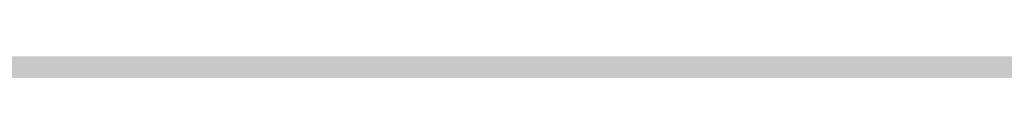
# Model space of a CAD drawing. Units: feet. Extents: x 3168 to 4724, y 827 to 1477.
# Tile 168 of 256: x 3301.945 to 3303.032, y 1099.001 to 1099.015. Entities that reach past the tile are written whole.
import ezdxf

# ---------------------------------------------------------------- set-up
doc = ezdxf.new("R2010")
doc.units = ezdxf.units.FT
doc.layers.add('A-ELEV', color=7, linetype='Continuous', lineweight=35)
doc.layers.add('A-ELEV-PATT', color=8, linetype='Continuous', lineweight=13)

msp = doc.modelspace()

# ---------------------------------------------------------------- hatches: boundary and pattern name
at = {"layer": 'A-ELEV-PATT'}
h = msp.add_hatch(color=256, dxfattribs=at)
h.dxf.hatch_style = 1
edge = h.paths.add_edge_path()
edge.add_ellipse((3552.9058, 979.2201), major_axis=(36.7449, 0), ratio=0.4848485, start_angle=0, end_angle=360)
edge = h.paths.add_edge_path()
edge.add_ellipse((3559.8916, 929.2523), major_axis=(36.7449, 0), ratio=0.4848485, start_angle=0, end_angle=360)
edge = h.paths.add_edge_path()
edge.add_line((3299.3168, 1198.6061), (3479.9167, 1198.6061))
edge.add_line((3479.9167, 1198.6061), (3479.9167, 1209.8686))
edge.add_spline(control_points=[(3479.9167, 1209.8686), (3464.3012, 1209.8686), (3448.6856, 1209.8686), (3410.9491, 1209.8686), (3388.8282, 1209.8686), (3355.6469, 1209.8686), (3344.5864, 1209.8686), (3327.9957, 1209.8686), (3322.4655, 1209.8686), (3314.1702, 1209.8686), (3311.4051, 1209.8686), (3307.2574, 1209.8686), (3305.8748, 1209.8686), (3303.801, 1209.8686), (3303.1097, 1209.8686), (3302.0728, 1209.8686), (3301.7272, 1209.8686), (3301.2087, 1209.8686), (3301.0359, 1209.8686), (3300.7767, 1209.8686), (3300.6903, 1209.8686), (3300.5606, 1209.8686), (3300.5174, 1209.8686), (3300.4526, 1209.8686), (3300.431, 1209.8686), (3300.3986, 1209.8686), (3300.3878, 1209.8686), (3300.3662, 1209.8686), (3300.3457, 1209.8686), (3300.3455, 1209.8686), (3300.3455, 1209.8686), (3300.3433, 1209.8686), (3300.3411, 1209.8686), (3300.3379, 1209.8686), (3300.3368, 1209.8686), (3300.3339, 1209.8686), (3300.3321, 1209.8686), (3300.3255, 1209.8686), (3300.3207, 1209.8686), (3300.3109, 1209.8686), (3300.306, 1209.8686), (3300.2905, 1209.8686), (3300.28, 1209.8686), (3300.2324, 1209.8688), (3300.1953, 1209.869), (3299.9511, 1209.8706), (3299.7448, 1209.8743), (3299.4368, 1209.8833), (3299.3344, 1209.8868), (3299.1811, 1209.8929), (3299.13, 1209.8951), (3298.6522, 1209.9168), (3298.2295, 1209.9457), (3297.6016, 1210.0024), (3297.3934, 1210.0235), (3297.0827, 1210.0583), (3296.9793, 1210.0705), (3296.293, 1210.1549), (3295.7181, 1210.2434), (3294.8687, 1210.3989), (3294.5877, 1210.4545), (3294.1693, 1210.5433), (3294.0304, 1210.5739), (3291.7071, 1211.1012), (3289.6536, 1211.8134), (3285.7763, 1213.564), (3283.9514, 1214.6035), (3280.5122, 1216.9801), (3278.8972, 1218.3176), (3276.3799, 1220.8295), (3275.416, 1221.9177), (3274.0393, 1223.7077), (3273.581, 1224.3495), (3273.1432, 1225.0163)], knot_values=[39.119033, 39.119033, 39.119033, 39.119033, 39.286353, 39.286353, 39.523379, 39.523379, 39.641892, 39.641892, 39.701148, 39.701148, 39.730777, 39.730777, 39.745591, 39.745591, 39.752998, 39.752998, 39.756701, 39.756701, 39.758553, 39.758553, 39.759479, 39.759479, 39.759942, 39.759942, 39.760173, 39.760173, 39.760289, 39.760289, 39.760405, 39.760405, 39.760463, 39.760463, 39.763389, 39.763389, 39.764851, 39.764851, 39.767304, 39.767304, 39.773825, 39.773825, 39.78057, 39.78057, 39.79477, 39.79477, 39.845194, 39.845194, 40.126715, 40.126715, 40.267476, 40.267476, 40.337856, 40.337856, 40.927023, 40.927023, 41.221606, 41.221606, 41.368898, 41.368898, 42.202622, 42.202622, 42.619485, 42.619485, 42.827916, 42.827916, 46.118323, 46.118323, 49.408731, 49.408731, 52.699139, 52.699139, 54.927489, 54.927489, 56.104228, 56.104228, 56.104228, 56.104228], weights=[1, 1, 1, 1, 1, 1, 1, 1, 1, 1, 1, 1, 1, 1, 1, 1, 1, 1, 1, 1, 1, 1, 1, 1, 1, 1, 1, 1, 1, 1, 1, 1, 1, 1, 1, 1, 1, 1, 1, 1, 1, 1, 1, 1, 1, 1, 1, 1, 1, 1, 1, 1, 1, 1, 1, 1, 1, 1, 1, 1, 1, 1, 1, 1, 1, 1, 1, 1, 1, 1, 1, 1, 1, 1], degree=3, periodic=0)
edge.add_line((3273.1432, 1225.0163), (3273.1432, 1099.0163))
edge.add_line((3273.1432, 1099.0163), (3299.3168, 1099.0163))
edge.add_line((3299.3168, 1099.0163), (3299.3168, 1198.6061))
edge = h.paths.add_edge_path()
edge.add_line((3304.7584, 1324.1581), (3479.9167, 1324.1581))
edge.add_line((3479.9167, 1324.1581), (3479.9167, 1335.7146))
edge.add_line((3479.9167, 1335.7146), (3269.1616, 1335.7146))
edge.add_spline(control_points=[(3269.1616, 1335.7146), (3264.0242, 1335.7146), (3258.3641, 1328.9582), (3259.2643, 1323.9003)], knot_values=[0, 0, 0, 0, 15.412191, 15.412191, 15.412191, 15.412191], degree=3, periodic=0)
edge.add_line((3259.2643, 1323.9003), (3265.5168, 1288.7691))
edge.add_line((3265.5168, 1288.7691), (3275.2651, 1261.5456))
edge.add_line((3275.2651, 1261.5456), (3304.7584, 1261.5456))
edge.add_line((3304.7584, 1261.5456), (3304.7584, 1324.1581))
h = msp.add_hatch(color=256, dxfattribs=at)
h.dxf.hatch_style = 1
h.paths.add_polyline_path([(3384.5252, 1099.0163), (3335.0292, 1099.0163), (3299.3168, 1099.0163), (3273.1432, 1099.0163), (3217.5654, 1099.0163), (3168.0693, 827.1163), (3335.0292, 827.1163)])

# ---------------------------------------------------------------- linework, layer by layer
at = {"layer": 'A-ELEV'}
msp.add_open_spline([(3808.5202, 1099.0163), (3808.5202, 1141.4132), (3808.5202, 1183.8102), (3808.5202, 1226.6353), (3808.5202, 1227.0636), (3808.5202, 1227.4918), (3811.4919, 1248.9947), (3814.4635, 1270.4975), (3817.4652, 1292.2176), (3817.4952, 1292.4348), (3817.5253, 1292.652), (3817.5728, 1310.1067), (3817.6203, 1327.5615), (3817.6679, 1345.0163), (3817.6679, 1345.458), (3817.6679, 1345.8996), (3817.6679, 1346.456), (3817.6679, 1346.5708), (3817.6679, 1346.7529), (3817.6679, 1346.8201), (3817.6679, 1346.9349), (3817.6679, 1346.9823), (3817.6679, 1347.0386), (3817.6679, 1347.0474), (3817.6679, 1347.0737), (3817.6679, 1347.0593), (3817.6679, 1347.0615), (3817.6679, 1347.0627), (3817.6679, 1347.066), (3817.6679, 1347.0683), (3817.6679, 1347.075), (3817.6679, 1347.0795), (3817.6678, 1347.0929), (3817.6678, 1347.1019), (3817.6678, 1347.1288), (3817.6677, 1347.1467), (3817.6674, 1347.2004), (3817.6672, 1347.2362), (3817.6661, 1347.3434), (3817.665, 1347.4147), (3817.6608, 1347.6281), (3817.6566, 1347.7697), (3817.64, 1348.1925), (3817.6235, 1348.4716), (3817.5591, 1349.3001), (3817.4961, 1349.8406), (3817.2554, 1351.4242), (3817.0263, 1352.4288), (3816.3069, 1354.8889), (3815.7437, 1356.2687), (3814.464, 1358.8192), (3813.7464, 1359.991), (3812.1958, 1362.1723), (3811.3622, 1363.1821), (3809.5888, 1365.069), (3808.6488, 1365.9461), (3806.6543, 1367.5796), (3805.5997, 1368.3362), (3803.3529, 1369.7223), (3802.1605, 1370.3524), (3799.6008, 1371.4536), (3798.2327, 1371.9255), (3795.2801, 1372.6346), (3793.6931, 1372.8721), (3791.8694, 1372.9265), (3791.7409, 1372.9292), (3791.3534, 1372.9341), (3791.0927, 1372.9329), (3790.3041, 1372.9151), (3789.7695, 1372.8842), (3789.2092, 1372.8302), (3789.1906, 1372.8284), (3789.1349, 1372.8229), (3789.0977, 1372.8191), (3789.0484, 1372.814), (3789.0364, 1372.8127), (3789.0003, 1372.8089), (3788.9761, 1372.8063), (3788.9494, 1372.8034), (3788.9468, 1372.8031), (3788.9426, 1372.8027), (3788.941, 1372.8025), (3788.9386, 1372.8022), (3788.9378, 1372.8021), (3788.9354, 1372.8019), (3788.8675, 1372.7944), (3788.7569, 1372.7822), (3788.7015, 1372.7761), (3788.5355, 1372.7579), (3788.4249, 1372.7457), (3788.0929, 1372.7092), (3787.8715, 1372.6848), (3787.2075, 1372.6118), (3786.7648, 1372.5631), (3785.4368, 1372.417), (3784.5515, 1372.3196), (3781.8954, 1372.0274), (3780.1247, 1371.8327), (3774.8126, 1371.2483), (3771.2713, 1370.8587), (3760.6471, 1369.69), (3753.5643, 1368.9109), (3732.316, 1366.5735), (3718.1504, 1365.0152), (3694.0068, 1362.3593), (3684.0287, 1361.2617), (3674.0506, 1360.1641), (3664.6007, 1360.1641), (3655.1508, 1360.1641), (3626.8011, 1360.1641), (3607.9013, 1360.1641), (3551.2019, 1360.1641), (3513.4023, 1360.1641), (3467.7252, 1360.1641), (3459.8476, 1360.1641), (3436.2149, 1360.1641), (3420.4597, 1360.1641), (3373.1943, 1360.1641), (3341.6839, 1360.1641), (3302.8482, 1360.1641), (3295.5227, 1360.1641), (3286.0383, 1360.1641), (3283.8794, 1360.1641), (3277.4026, 1360.1641), (3273.0848, 1360.1641), (3267.7329, 1360.1641), (3266.6988, 1360.1641), (3263.5965, 1360.1641), (3261.5284, 1360.1641), (3259.2369, 1360.1641), (3259.0137, 1360.1641), (3258.344, 1360.1641), (3257.8975, 1360.1641), (3257.431, 1360.1641), (3257.411, 1360.1641), (3257.3706, 1360.1641), (3257.3755, 1360.1641), (3257.3746, 1360.1641), (3257.3739, 1360.1641), (3257.372, 1360.1641), (3257.3706, 1360.1641), (3257.3667, 1360.1641), (3257.364, 1360.1641), (3257.3561, 1360.1641), (3257.3508, 1360.164), (3257.335, 1360.164), (3257.3244, 1360.164), (3257.2928, 1360.1639), (3257.2717, 1360.1638), (3257.2084, 1360.1634), (3257.1663, 1360.163), (3257.0402, 1360.1614), (3256.9563, 1360.1598), (3256.7055, 1360.1534), (3256.5392, 1360.147), (3256.0436, 1360.1219), (3255.7173, 1360.0971), (3254.7524, 1360.0005), (3254.128, 1359.9065), (3252.1801, 1359.5253), (3250.9416, 1359.144), (3248.6702, 1358.2433), (3247.6357, 1357.7238), (3245.7326, 1356.6035), (3244.8634, 1356.0021), (3243.2531, 1354.7429), (3242.512, 1354.0847), (3240.7511, 1352.3448), (3239.801, 1351.2296), (3238.0878, 1348.8724), (3237.3247, 1347.6304), (3235.9825, 1344.9716), (3235.4022, 1343.5549), (3234.5911, 1340.8155), (3234.3109, 1339.5435), (3233.9765, 1336.8026), (3233.9221, 1335.3309), (3234.1489, 1332.5913), (3234.3495, 1331.3672), (3234.7199, 1329.9994), (3234.7524, 1329.8834), (3234.8536, 1329.5348), (3234.9259, 1329.3017), (3235.0248, 1329.0026), (3235.0469, 1328.9369), (3235.0776, 1328.8472), (3235.0859, 1328.8232), (3235.1109, 1328.7511), (3235.1278, 1328.703), (3235.148, 1328.6462), (3235.1511, 1328.6376), (3235.1561, 1328.6235), (3235.1581, 1328.618), (3235.1602, 1328.612), (3235.1656, 1328.5969), (3235.1801, 1328.5565), (3235.1903, 1328.5281), (3235.2208, 1328.4429), (3235.2411, 1328.3862), (3235.3021, 1328.2159), (3235.3427, 1328.1023), (3235.4647, 1327.7617), (3235.546, 1327.5346), (3235.79, 1326.8534), (3235.9526, 1326.3992), (3236.4405, 1325.0367), (3236.7657, 1324.1284), (3237.7415, 1321.4034), (3238.392, 1319.5868), (3240.3435, 1314.1369), (3241.6445, 1310.5036), (3245.5476, 1299.6037), (3248.1496, 1292.3371), (3255.9557, 1270.5374), (3261.1598, 1256.0042), (3267.3876, 1238.612), (3268.4114, 1235.7529), (3269.5104, 1232.6839), (3269.5856, 1232.4739), (3269.7066, 1232.1359), (3269.7524, 1232.0079), (3269.8273, 1231.7987), (3269.8564, 1231.7176), (3269.9063, 1231.5781), (3269.9272, 1231.5198), (3269.9725, 1231.3934), (3269.9968, 1231.3254), (3270.0265, 1231.2425), (3270.0318, 1231.2277), (3270.0403, 1231.204), (3270.0392, 1231.207), (3270.0394, 1231.2066), (3270.0394, 1231.2064), (3270.0396, 1231.2058), (3270.0398, 1231.2055), (3270.0402, 1231.2043), (3270.0404, 1231.2036), (3270.0413, 1231.2013), (3270.0418, 1231.1998), (3270.0434, 1231.1953), (3270.0445, 1231.1922), (3270.0478, 1231.1832), (3270.0499, 1231.1771), (3270.0564, 1231.159), (3270.0608, 1231.147), (3270.0739, 1231.1108), (3270.0826, 1231.0867), (3270.1089, 1231.0144), (3270.1266, 1230.9663), (3270.1799, 1230.8225), (3270.2159, 1230.7269), (3270.3253, 1230.4415), (3270.4, 1230.2528), (3270.6292, 1229.6914), (3270.7889, 1229.3235), (3271.2865, 1228.2383), (3271.6431, 1227.5398), (3272.7759, 1225.5153), (3273.6142, 1224.2605), (3275.416, 1221.9177), (3276.3799, 1220.8295), (3278.8972, 1218.3176), (3280.5122, 1216.9801), (3283.9514, 1214.6035), (3285.7763, 1213.564), (3289.6536, 1211.8134), (3291.7071, 1211.1012), (3294.0304, 1210.5739), (3294.1693, 1210.5433), (3294.5877, 1210.4545), (3294.8687, 1210.3989), (3295.7181, 1210.2434), (3296.293, 1210.1549), (3296.9793, 1210.0705), (3297.0827, 1210.0583), (3297.3934, 1210.0235), (3297.6016, 1210.0024), (3298.2295, 1209.9457), (3298.6522, 1209.9168), (3299.13, 1209.8951), (3299.1811, 1209.8929), (3299.3344, 1209.8868), (3299.4368, 1209.8833), (3299.7448, 1209.8743), (3299.9511, 1209.8706), (3300.1953, 1209.869), (3300.2324, 1209.8688), (3300.28, 1209.8686), (3300.2905, 1209.8686), (3300.306, 1209.8686), (3300.3109, 1209.8686), (3300.3207, 1209.8686), (3300.3255, 1209.8686), (3300.3321, 1209.8686), (3300.3339, 1209.8686), (3300.3368, 1209.8686), (3300.3379, 1209.8686), (3300.3411, 1209.8686), (3300.3433, 1209.8686), (3300.3455, 1209.8686), (3300.3455, 1209.8686), (3300.3457, 1209.8686), (3300.3662, 1209.8686), (3300.3878, 1209.8686), (3300.3986, 1209.8686), (3300.431, 1209.8686), (3300.4526, 1209.8686), (3300.5174, 1209.8686), (3300.5606, 1209.8686), (3300.6903, 1209.8686), (3300.7767, 1209.8686), (3301.0359, 1209.8686), (3301.2087, 1209.8686), (3301.7272, 1209.8686), (3302.0728, 1209.8686), (3303.1097, 1209.8686), (3303.801, 1209.8686), (3305.8748, 1209.8686), (3307.2574, 1209.8686), (3311.4051, 1209.8686), (3314.1702, 1209.8686), (3322.4655, 1209.8686), (3327.9957, 1209.8686), (3344.5864, 1209.8686), (3355.6469, 1209.8686), (3388.8282, 1209.8686), (3410.9491, 1209.8686), (3477.3119, 1209.8686), (3521.5537, 1209.8686), (3566.8362, 1209.8686), (3567.8769, 1209.8686), (3570.999, 1209.8686), (3573.0804, 1209.8686), (3575.7814, 1209.8686), (3576.4009, 1209.8686), (3577.2958, 1209.8686), (3577.5712, 1209.8686), (3578.3971, 1209.8686), (3578.9478, 1209.8686), (3579.7565, 1209.8686), (3580.0145, 1209.8686), (3580.3427, 1209.8686), (3580.3269, 1209.8686), (3580.3272, 1209.8686), (3580.3273, 1209.8686), (3580.3278, 1209.8686), (3580.3281, 1209.8686), (3580.329, 1209.8686), (3580.3296, 1209.8686), (3580.3314, 1209.8686), (3580.3327, 1209.8686), (3580.3363, 1209.8686), (3580.3388, 1209.8686), (3580.3461, 1209.8686), (3580.351, 1209.8686), (3580.3657, 1209.8685), (3580.3754, 1209.8685), (3580.4048, 1209.8684), (3580.4244, 1209.8684), (3580.4832, 1209.8681), (3580.5224, 1209.8678), (3580.6404, 1209.8666), (3580.7192, 1209.8655), (3580.9563, 1209.8608), (3581.1152, 1209.8561), (3581.5942, 1209.8372), (3581.9164, 1209.8183), (3582.8899, 1209.7424), (3583.548, 1209.6662), (3585.5318, 1209.3606), (3586.8672, 1209.0539), (3589.4715, 1208.2525), (3590.7402, 1207.7579), (3591.9955, 1207.1588), (3592.0578, 1207.1287), (3592.2442, 1207.038), (3592.3677, 1206.9766), (3592.7353, 1206.7904), (3592.9768, 1206.6631), (3593.2445, 1206.5164), (3593.2747, 1206.4998), (3593.3651, 1206.4498), (3593.4251, 1206.4163), (3593.6043, 1206.3153), (3593.7227, 1206.2472), (3593.8572, 1206.1684), (3593.8744, 1206.1583), (3593.9257, 1206.128), (3593.9599, 1206.1078), (3594.0621, 1206.0469), (3594.1298, 1206.0061), (3594.2084, 1205.9582), (3594.2197, 1205.9513), (3594.2534, 1205.9307), (3594.2758, 1205.9169), (3594.343, 1205.8755), (3594.3876, 1205.8479), (3594.4336, 1205.819), (3594.4353, 1205.818), (3594.4402, 1205.8149), (3594.4435, 1205.8129), (3594.4471, 1205.8106), (3594.4475, 1205.8103), (3594.4487, 1205.8096), (3594.4495, 1205.8091), (3594.4504, 1205.8086), (3594.4505, 1205.8085), (3594.4506, 1205.8084), (3594.4674, 1205.7979), (3594.4933, 1205.7817), (3594.5062, 1205.7736), (3594.545, 1205.7492), (3594.5709, 1205.733), (3594.6485, 1205.6844), (3594.7002, 1205.652), (3594.8554, 1205.5547), (3594.9589, 1205.4898), (3595.2694, 1205.2953), (3595.4763, 1205.1656), (3596.0972, 1204.7765), (3596.5111, 1204.5171), (3597.7528, 1203.7388), (3598.5807, 1203.22), (3601.0642, 1201.6636), (3602.7198, 1200.6259), (3607.6868, 1197.513), (3610.9981, 1195.4377), (3620.932, 1189.2119), (3627.5546, 1185.0614), (3647.4225, 1172.6097), (3660.6678, 1164.3086), (3700.4035, 1139.4053), (3726.894, 1122.8031), (3757.2057, 1103.8061), (3761.027, 1101.4112), (3764.8482, 1099.0163), (3745.3283, 1099.0163), (3725.8083, 1099.0163), (3706.2884, 1099.0163), (3706.2884, 1108.4532), (3706.2884, 1117.8902), (3706.2884, 1127.3271), (3710.7508, 1127.3271), (3715.2131, 1127.3271), (3719.6755, 1127.3271)], degree=3, knots=[0, 0, 0, 0, 0.982037, 0.982037, 0.991957, 0.991957, 0.991957, 1.966522, 1.966522, 1.976367, 1.976367, 1.976367, 2.976367, 2.976367, 2.976367, 3.00169, 3.00169, 3.008272, 3.008272, 3.012129, 3.012129, 3.014851, 3.014851, 3.015353, 3.015353, 3.016359, 3.016359, 3.017365, 3.017365, 3.019376, 3.019376, 3.023398, 3.023398, 3.031442, 3.031442, 3.047531, 3.047531, 3.079708, 3.079708, 3.144063, 3.144063, 3.272772, 3.272772, 3.53019, 3.53019, 4.045026, 4.045026, 5.074698, 5.074698, 6.700878, 6.700878, 8.327058, 8.327058, 9.953238, 9.953238, 11.579418, 11.579418, 13.205598, 13.205598, 14.831778, 14.831778, 16.457958, 16.457958, 18.084138, 18.084138, 18.206872, 18.206872, 18.45234, 18.45234, 18.943275, 18.943275, 18.960093, 18.960093, 18.993729, 18.993729, 19.00461, 19.00461, 19.026374, 19.026374, 19.028737, 19.028737, 19.03018, 19.03018, 19.030897, 19.030897, 19.032332, 19.032332, 19.033766, 19.033766, 19.036636, 19.036636, 19.042374, 19.042374, 19.053851, 19.053851, 19.076805, 19.076805, 19.122714, 19.122714, 19.21453, 19.21453, 19.398163, 19.398163, 19.765429, 19.765429, 20.024128, 20.024128, 20.024128, 20.092031, 20.092031, 20.227836, 20.227836, 20.499446, 20.499446, 20.556051, 20.556051, 20.66926, 20.66926, 20.895678, 20.895678, 20.948316, 20.948316, 20.963829, 20.963829, 20.994855, 20.994855, 21.002285, 21.002285, 21.017146, 21.017146, 21.01875, 21.01875, 21.021959, 21.021959, 21.022102, 21.022102, 21.022249, 21.022249, 21.022708, 21.022708, 21.023627, 21.023627, 21.025464, 21.025464, 21.029138, 21.029138, 21.036486, 21.036486, 21.051183, 21.051183, 21.080575, 21.080575, 21.139361, 21.139361, 21.256932, 21.256932, 21.492073, 21.492073, 21.962356, 21.962356, 23.01002, 23.01002, 24.057684, 24.057684, 25.105348, 25.105348, 26.153011, 26.153011, 27.776787, 27.776787, 29.400562, 29.400562, 31.024337, 31.024337, 32.278801, 32.278801, 33.533265, 33.533265, 34.467568, 34.467568, 34.553971, 34.553971, 34.726776, 34.726776, 34.775309, 34.775309, 34.793079, 34.793079, 34.82862, 34.82862, 34.834979, 34.834979, 34.839039, 34.839039, 34.839411, 34.839411, 34.840285, 34.840285, 34.842034, 34.842034, 34.845531, 34.845531, 34.852525, 34.852525, 34.866512, 34.866512, 34.894488, 34.894488, 34.950439, 34.950439, 35.062342, 35.062342, 35.286147, 35.286147, 35.733758, 35.733758, 35.821815, 35.821815, 35.828283, 35.828283, 35.832225, 35.832225, 35.834724, 35.834724, 35.836521, 35.836521, 35.838617, 35.838617, 35.839073, 35.839073, 35.839345, 35.839345, 35.839617, 35.839617, 35.840161, 35.840161, 35.841249, 35.841249, 35.843425, 35.843425, 35.847778, 35.847778, 35.856482, 35.856482, 35.873891, 35.873891, 35.908709, 35.908709, 35.978345, 35.978345, 36.117617, 36.117617, 36.396161, 36.396161, 36.953248, 36.953248, 38.067423, 38.067423, 40.295772, 40.295772, 42.524122, 42.524122, 45.81453, 45.81453, 49.104937, 49.104937, 52.395345, 52.395345, 52.603776, 52.603776, 53.020639, 53.020639, 53.854363, 53.854363, 54.001655, 54.001655, 54.296238, 54.296238, 54.885405, 54.885405, 54.955785, 54.955785, 55.096546, 55.096546, 55.378067, 55.378067, 55.42849, 55.42849, 55.442691, 55.442691, 55.449436, 55.449436, 55.455957, 55.455957, 55.458409, 55.458409, 55.459872, 55.459872, 55.462798, 55.462798, 55.462856, 55.462856, 55.462972, 55.462972, 55.463088, 55.463088, 55.463319, 55.463319, 55.463782, 55.463782, 55.464708, 55.464708, 55.46656, 55.46656, 55.470263, 55.470263, 55.47767, 55.47767, 55.492484, 55.492484, 55.522112, 55.522112, 55.581369, 55.581369, 55.699882, 55.699882, 55.936907, 55.936907, 56.410959, 56.410959, 56.42211, 56.42211, 56.444413, 56.444413, 56.451051, 56.451051, 56.454001, 56.454001, 56.459901, 56.459901, 56.462666, 56.462666, 56.463418, 56.463418, 56.464171, 56.464171, 56.465675, 56.465675, 56.468684, 56.468684, 56.474702, 56.474702, 56.486738, 56.486738, 56.51081, 56.51081, 56.558955, 56.558955, 56.655243, 56.655243, 56.847821, 56.847821, 57.232975, 57.232975, 58.003284, 58.003284, 59.543901, 59.543901, 62.625137, 62.625137, 68.787607, 68.787607, 74.950078, 74.950078, 75.27336, 75.27336, 75.919923, 75.919923, 77.213051, 77.213051, 77.377769, 77.377769, 77.707206, 77.707206, 78.366079, 78.366079, 78.462532, 78.462532, 78.655436, 78.655436, 79.041245, 79.041245, 79.105735, 79.105735, 79.234714, 79.234714, 79.492672, 79.492672, 79.502197, 79.502197, 79.521249, 79.521249, 79.523534, 79.523534, 79.528103, 79.528103, 79.528682, 79.528682, 79.528885, 79.528885, 79.529089, 79.529089, 79.529495, 79.529495, 79.530308, 79.530308, 79.531935, 79.531935, 79.535187, 79.535187, 79.541693, 79.541693, 79.554704, 79.554704, 79.580725, 79.580725, 79.632769, 79.632769, 79.736856, 79.736856, 79.94503, 79.94503, 80.361377, 80.361377, 80.421435, 80.421435, 80.421435, 81.421435, 81.421435, 81.421435, 82.421435, 82.421435, 82.421435, 83.421435, 83.421435, 83.421435, 83.421435], dxfattribs=at)

doc.saveas('drawing.dxf')
